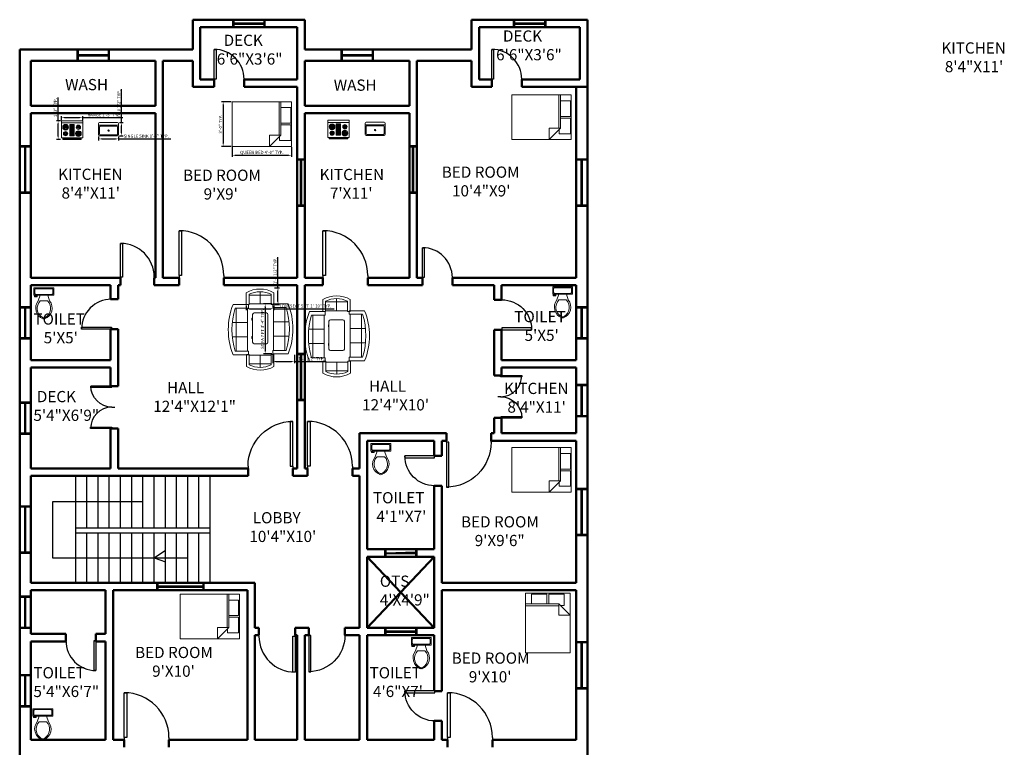
# Model space of a CAD drawing. Units: inches. Extents: x -31438 to -28352, y 12489 to 13610.
# Tile 5 of 5: x -29143 to -28352, y 13026 to 13610. Entities that reach past the tile are written whole.
import ezdxf

# ---------------------------------------------------------------- set-up
doc = ezdxf.new("R2010")
doc.units = ezdxf.units.IN
for name, color, linetype, lineweight in [('A-ANNO-DIMS', 2, 'Continuous', 18), ('A-AREA-IDEN', 3, 'Continuous', 18), ('A-DOOR', 3, 'Continuous', 25), ('A-FLOR-FIXT', 9, 'Continuous', 18), ('A-FLOR-STRS', 6, 'Continuous', 25), ('A-FURN', 8, 'Continuous', 18), ('A-GLAZ', 4, 'Continuous', 25), ('A-WALL', 7, 'Continuous', 50)]:
    doc.layers.add(name, color=color, linetype=linetype, lineweight=lineweight)
doc.styles.get("Standard").update_dxf_attribs({"font": 'arial.ttf'})
doc.dimstyles.new('ISO-25', dxfattribs={"dimtxt": 2.5, "dimasz": 2.5, "dimexe": 1.25, "dimexo": 0.625, "dimtad": 1, "dimdec": 0, "dimlunit": 3, "dimtxsty": 'Standard', "dimcen": 2.5, "dimadec": 0, "dimazin": 0, "dimtfac": 1, "dimtdec": 0, "dimtmove": 0, "dimatfit": 3, "dimfxl": 1, "dimarcsym": 0})

# ---------------------------------------------------------------- blocks, each defined once
blk = doc.blocks.new('*U8')
for p, q in [((0, 0), (0, -100)), ((750, 0), (750, -100))]:
    blk.add_line(p, q)
blk.add_lwpolyline([(0, 0), (0, 750), (43.75, 750), (43.75, 0)], close=True)
blk.add_arc((0, 0), 750, 0, 90)
blk = doc.blocks.new('Bed - Queen')
for p, q in [((0, -80.00003), (0, 0)), ((0, 0), (59.99999, 0)), ((59.99999, 0), (59.99999, -80.00003)), ((7.99999, -1.2), (28.79998, -1.2)), ((7.99999, -14.4), (7.99999, -1.2)), ((28.79998, -1.2), (28.79998, -14.4)), ((31.19999, -1.2), (51.99999, -1.2)), ((31.19999, -14.4), (31.19999, -1.2)), ((51.99999, -1.2), (51.99999, -16.4)), ((0, -14.4), (44.8, -14.4)), ((44.8, -16.8), (0, -16.8)), ((59.99999, -29.6), (44.8, -14.4)), ((44.8, -14.4), (44.8, -29.6)), ((51.99999, -16.4), (46.79936, -16.4)), ((44.8, -29.6), (59.99999, -29.6)), ((59.99999, -80.00003), (0, -80.00003))]:
    blk.add_line(p, q)
blk = doc.blocks.new('Desk - 30 x 60 in.')
for p, q in [((-26.999995, 0), (26.999995, 0)), ((-29.999995, -27), (-29.999995, -3)), ((29.999995, -3), (29.999995, -27)), ((26.999995, -30), (-26.999995, -30)), ((-20.000005, -30), (-20.000005, -31)), ((-20.000005, -31), (-16.000005, -31)), ((-16.000005, -31), (-16.000005, -30)), ((15.999995, -31), (15.999995, -30)), ((19.999995, -31), (15.999995, -31)), ((19.999995, -30), (19.999995, -31))]:
    blk.add_line(p, q)
for centre, start, end in [((-26.499995, -3.5), 98.1301, 171.8699), ((26.499995, -3.5), 8.130102, 81.8699), ((-26.499995, -26.5), 188.1301, 261.8699), ((26.499995, -26.5), 278.1301, 351.8699)]:
    blk.add_arc(centre, 3.535534, start, end)
blk = doc.blocks.new('Sofa - Roundback 7 ft.')
for p, q in [((-36.000027, -34), (-36.000027, -11.4696)), ((-35.999844, -13.3819), (35.9998, -13.3819)), ((-12.00002, -32.4421), (-12.00003, -6.5971)), ((11.99997, -32.4421), (11.99998, -6.5971)), ((35.99998, -34), (35.99998, -11.4696)), ((-36.000027, -32.4421), (35.99998, -32.4421))]:
    blk.add_line(p, q)
for points in [[(-36.000027, -34), (-42.000027, -34), (-42.000027, -8)], [(41.99998, -8), (41.99998, -34), (35.99998, -34)]]:
    blk.add_lwpolyline(points)
for centre, radius, start, end in [((0, -114.25), 114.25, 68.43141, 111.5686), ((-0.00001, -127.1968), 121.1968, 72.72033, 107.2797)]:
    blk.add_arc(centre, radius, start, end)
blk = doc.blocks.new('Sofa - Roundback Loveseat 5 ft.')
for p, q in [((-24, -33.99998), (-24, -11.46958)), ((-23.9998, -13.38178), (23.99986, -13.38178)), ((0, -32.44198), (0, -5.99998)), ((24.00004, -33.99998), (24.00004, -11.46958)), ((-24, -32.44198), (24.00004, -32.44198))]:
    blk.add_line(p, q)
for points in [[(-24, -33.99998), (-30, -33.99998), (-30, -7.99998)], [(30.00004, -7.99998), (30.00004, -33.99998), (24.00004, -33.99998)]]:
    blk.add_lwpolyline(points)
for centre, radius, start, end in [((0, -60.24998), 60.24998, 60.13715, 119.8628), ((0, -61.38438), 55.38444, 64.32083, 115.6792)]:
    blk.add_arc(centre, radius, start, end)
blk = doc.blocks.new('Toilet - top')
for p, q in [((-10, -8.5), (-8, -8.5)), ((-10, -9.5), (-10, -8.5)), ((-7, -9.5), (-10, -9.5)), ((-8, -8.5), (-8, -8)), ((-7, -8), (-7, -9.5)), ((-4, -8), (-6, -14)), ((4, -8), (6, -14)), ((9.5, -6), (9.5, -2)), ((4, -14), (-4, -14))]:
    blk.add_line(p, q)
blk.add_lwpolyline([(10.5, -8), (10.5, 0), (-10.5, 0), (-10.5, -8)], close=True)
for points in [[(-9.5, -2), (-9.5, -6)], [(8.5, -1), (-8.5, -1)], [(-8.5, -7), (8.5, -7)]]:
    blk.add_lwpolyline(points)
for centre, radius, start, end in [((-8.6, -1.9), 0.884, 81.8699, 188.1301), ((-8.6, -6.1), 0.884, 171.8699, 278.1301), ((8.6, -1.9), 0.884, 351.8699, 98.1301), ((8.6, -6.1), 0.884, 261.8699, 8.1301), ((3.5, -21.6), 12.2, 141.4691, 247.9714), ((4.2, -21.8), 11.3, 136.3677, 238.9468), ((-3.5, -21.6), 12.2, 292.0284, 38.5307), ((-4.2, -21.8), 11.3, 301.053, 43.6321), ((0, -27.9), 4, 245.7318, 294.2682), ((0, -29), 4, 254.8605, 285.1395)]:
    blk.add_arc(centre, radius, start, end)
blk = doc.blocks.new('Range-Oven - 30 in top')
for p, q in [((0, -3), (30, -3)), ((12, -6), (18, -6)), ((13, -20), (13, -6)), ((14, -6), (14, -20)), ((15, -20), (15, -6)), ((16, -6), (16, -20)), ((17, -20), (17, -6)), ((6, -24), (6, -25)), ((8, -25), (8, -24)), ((18, -20), (12, -20)), ((22, -25), (22, -24)), ((24, -24), (24, -25))]:
    blk.add_line(p, q)
for points in [[(0, -24), (0, 0), (30, 0), (30, -24)], [(12, -21), (12, -5), (18, -5), (18, -21)], [(2, -26), (2, -25), (28, -25), (28, -26)]]:
    blk.add_lwpolyline(points, close=True)
for centre, radius in [((6, -9), 4), ((6, -9), 3), ((6, -9), 2), ((6, -9), 1), ((24, -9), 3), ((24, -9), 2), ((24, -9), 1), ((6, -18), 3), ((6, -18), 2), ((6, -18), 1), ((24, -18), 4), ((24, -18), 3), ((24, -18), 2), ((24, -18), 1)]:
    blk.add_circle(centre, radius)
blk = doc.blocks.new('Sink-single - 30 in top')
blk.add_line((-15, -3.999996), (15, -3.999996))
for points in [[(-13.5, 0), (13.5, 0)], [(-15, -18.499996), (-15, -1.5)], [(-13.5, -17.499996), (-13.5, -6.499996)], [(-12.5, -5.499996), (12.5, -5.499996)], [(13.5, -6.499996), (13.5, -17.499996)], [(15, -1.5), (15, -18.499996)], [(13.5, -19.999996), (-13.5, -19.999996)], [(12.5, -18.499996), (-12.5, -18.499996)]]:
    blk.add_lwpolyline(points)
for radius in [1, 0.5]:
    blk.add_circle((0, -11.999996), radius)
for centre, radius, start, end in [((-13.5, -1.5), 1.5, 90, 180), ((-12.5, -6.499996), 1, 90, 180), ((12.5, -6.499996), 1, 0, 90), ((13.5, -1.5), 1.5, 0, 90), ((-13.5, -18.499996), 1.5, 180, 270), ((-12.5, -17.499996), 1, 180, 270), ((12.5, -17.499996), 1, 270, 0), ((13.5, -18.499996), 1.5, 270, 0)]:
    blk.add_arc(centre, radius, start, end)
blk = doc.blocks.new('WIN-24')
for p, q in [((0, 0), (0, 24)), ((0.5, 0), (0.5, 24))]:
    blk.add_line(p, q)
blk = doc.blocks.new('WIN-36')
for p, q in [((0, 0), (0, 36)), ((0.5, 0), (0.5, 36))]:
    blk.add_line(p, q)
blk = doc.blocks.new('*D179')
at = {"layer": 'A-ANNO-DIMS', "color": 0, "lineweight": -2, "transparency": 16777216}
for p, q in [((-28940.39, 13381.63), (-28947.04, 13381.63)), ((-28945.79, 13379.13), (-28945.79, 13343.94)), ((-28940.39, 13341.44), (-28947.04, 13341.44))]:
    blk.add_line(p, q, dxfattribs=at)
at = {"layer": 'A-ANNO-DIMS', "color": 0, "transparency": 16777216}
for points in [[(-28946.21, 13379.13), (-28945.38, 13379.13), (-28945.79, 13381.63)], [(-28946.21, 13343.94), (-28945.38, 13343.94), (-28945.79, 13341.44)]]:
    blk.add_solid(points, dxfattribs=at)
at = {"layer": 'Defpoints', "color": 0, "transparency": 16777216}
for p in [(-28939.77, 13381.63), (-28945.79, 13341.44), (-28939.77, 13341.44)]:
    blk.add_point(p, dxfattribs=at)
at = {"layer": 'A-ANNO-DIMS', "color": 0, "transparency": 16777216, "insert": (-28947.71, 13361.54), "char_height": 2.5, "attachment_point": 5, "rotation": 90}
blk.add_mtext('SOFA 7 FT 3\'-4" TYP.', dxfattribs=at)
blk = doc.blocks.new('*D180')
at = {"layer": 'A-ANNO-DIMS', "color": 0, "lineweight": -2, "transparency": 16777216}
for p, q in [((-28939.77, 13340.82), (-28939.77, 13334.17)), ((-28937.27, 13335.42), (-28924.73, 13335.42)), ((-28922.23, 13340.82), (-28922.23, 13334.17)), ((-28922.23, 13335.42), (-28897.65, 13335.42))]:
    blk.add_line(p, q, dxfattribs=at)
at = {"layer": 'A-ANNO-DIMS', "color": 0, "transparency": 16777216}
for points in [[(-28937.27, 13335.83), (-28937.27, 13335), (-28939.77, 13335.42)], [(-28924.73, 13335.83), (-28924.73, 13335), (-28922.23, 13335.42)]]:
    blk.add_solid(points, dxfattribs=at)
at = {"layer": 'Defpoints', "color": 0, "transparency": 16777216}
for p in [(-28939.77, 13341.44), (-28922.23, 13341.44), (-28922.23, 13335.42)]:
    blk.add_point(p, dxfattribs=at)
at = {"layer": 'A-ANNO-DIMS', "color": 0, "transparency": 16777216, "insert": (-28908.69, 13337.33), "char_height": 2.5, "attachment_point": 5}
blk.add_mtext('1\'-5 1/2" TYP.', dxfattribs=at)
blk = doc.blocks.new('*D183')
at = {"layer": 'A-ANNO-DIMS', "color": 0, "lineweight": -2, "transparency": 16777216}
for p, q in [((-28960.97, 13380.44), (-28960.97, 13376.5)), ((-28958.47, 13377.75), (-28941.37, 13377.75)), ((-28938.87, 13380.44), (-28938.87, 13376.5)), ((-28938.87, 13377.75), (-28890.49, 13377.75))]:
    blk.add_line(p, q, dxfattribs=at)
at = {"layer": 'A-ANNO-DIMS', "color": 0, "transparency": 16777216}
for points in [[(-28958.47, 13378.17), (-28958.47, 13377.33), (-28960.97, 13377.75)], [(-28941.37, 13378.17), (-28941.37, 13377.33), (-28938.87, 13377.75)]]:
    blk.add_solid(points, dxfattribs=at)
at = {"layer": 'Defpoints', "color": 0, "transparency": 16777216}
for p in [(-28960.97, 13381.06), (-28938.87, 13381.06), (-28938.87, 13377.75)]:
    blk.add_point(p, dxfattribs=at)
at = {"layer": 'A-ANNO-DIMS', "color": 0, "transparency": 16777216, "insert": (-28913.43, 13379.67), "char_height": 2.5, "attachment_point": 5}
blk.add_mtext('LOVESEAT 5 FT 1\'-10" TYP.', dxfattribs=at)
blk = doc.blocks.new('*D184')
at = {"layer": 'A-ANNO-DIMS', "color": 0, "lineweight": -2, "transparency": 16777216}
for p, q in [((-28935.56, 13394.57), (-28935.56, 13419.14)), ((-28938.25, 13394.57), (-28934.31, 13394.57)), ((-28935.56, 13383.56), (-28935.56, 13392.07)), ((-28938.25, 13381.06), (-28934.31, 13381.06))]:
    blk.add_line(p, q, dxfattribs=at)
at = {"layer": 'A-ANNO-DIMS', "color": 0, "transparency": 16777216}
for points in [[(-28935.98, 13392.07), (-28935.14, 13392.07), (-28935.56, 13394.57)], [(-28935.98, 13383.56), (-28935.14, 13383.56), (-28935.56, 13381.06)]]:
    blk.add_solid(points, dxfattribs=at)
at = {"layer": 'Defpoints', "color": 0, "transparency": 16777216}
for p in [(-28938.87, 13394.57), (-28935.56, 13394.57), (-28938.87, 13381.06)]:
    blk.add_point(p, dxfattribs=at)
at = {"layer": 'A-ANNO-DIMS', "color": 0, "transparency": 16777216, "insert": (-28937.48, 13408.11), "char_height": 2.5, "attachment_point": 5, "rotation": 90}
blk.add_mtext('1\'-1 1/2" TYP.', dxfattribs=at)
blk = doc.blocks.new('*D187')
at = {"layer": 'A-ANNO-DIMS', "color": 0, "lineweight": -2, "transparency": 16777216}
for p, q in [((-28972.38, 13507.49), (-28972.38, 13499.69)), ((-28969.88, 13500.94), (-28927.09, 13500.94)), ((-28924.59, 13507.49), (-28924.59, 13499.69))]:
    blk.add_line(p, q, dxfattribs=at)
at = {"layer": 'A-ANNO-DIMS', "color": 0, "transparency": 16777216}
for points in [[(-28969.88, 13501.36), (-28969.88, 13500.53), (-28972.38, 13500.94)], [(-28927.09, 13501.36), (-28927.09, 13500.53), (-28924.59, 13500.94)]]:
    blk.add_solid(points, dxfattribs=at)
at = {"layer": 'Defpoints', "color": 0, "transparency": 16777216}
for p in [(-28972.38, 13508.11), (-28924.59, 13508.11), (-28924.59, 13500.94)]:
    blk.add_point(p, dxfattribs=at)
at = {"layer": 'A-ANNO-DIMS', "color": 0, "transparency": 16777216, "insert": (-28948.48, 13502.94), "char_height": 2.5, "attachment_point": 5}
blk.add_mtext('QUEEN BED 4\'-0" TYP.', dxfattribs=at)
blk = doc.blocks.new('*D188')
at = {"layer": 'A-ANNO-DIMS', "color": 0, "lineweight": -2, "transparency": 16777216}
for p, q in [((-28973, 13543.95), (-28980.8, 13543.95)), ((-28979.55, 13541.45), (-28979.55, 13510.61)), ((-28973, 13508.11), (-28980.8, 13508.11))]:
    blk.add_line(p, q, dxfattribs=at)
at = {"layer": 'A-ANNO-DIMS', "color": 0, "transparency": 16777216}
for points in [[(-28979.96, 13541.45), (-28979.13, 13541.45), (-28979.55, 13543.95)], [(-28979.96, 13510.61), (-28979.13, 13510.61), (-28979.55, 13508.11)]]:
    blk.add_solid(points, dxfattribs=at)
at = {"layer": 'Defpoints', "color": 0, "transparency": 16777216}
for p in [(-28972.38, 13543.95), (-28979.55, 13508.11), (-28972.38, 13508.11)]:
    blk.add_point(p, dxfattribs=at)
at = {"layer": 'A-ANNO-DIMS', "color": 0, "transparency": 16777216, "insert": (-28981.45, 13526.03), "char_height": 2.5, "attachment_point": 5, "rotation": 90}
blk.add_mtext('3\'-0" TYP.', dxfattribs=at)
blk = doc.blocks.new('*D199')
at = {"layer": 'A-ANNO-DIMS', "color": 0, "lineweight": -2, "transparency": 16777216}
for p, q in [((-29109.53, 13529.21), (-29109.53, 13532.4)), ((-29092.38, 13529.21), (-29092.38, 13532.4)), ((-29107.03, 13531.15), (-29094.88, 13531.15)), ((-29092.38, 13531.15), (-29060.13, 13531.15))]:
    blk.add_line(p, q, dxfattribs=at)
at = {"layer": 'A-ANNO-DIMS', "color": 0, "transparency": 16777216}
for points in [[(-29107.03, 13531.57), (-29107.03, 13530.74), (-29109.53, 13531.15)], [(-29094.88, 13531.57), (-29094.88, 13530.74), (-29092.38, 13531.15)]]:
    blk.add_solid(points, dxfattribs=at)
at = {"layer": 'Defpoints', "color": 0, "transparency": 16777216}
for p in [(-29109.53, 13528.58), (-29092.38, 13531.15), (-29092.38, 13528.58)]:
    blk.add_point(p, dxfattribs=at)
at = {"layer": 'A-ANNO-DIMS', "color": 0, "transparency": 16777216, "insert": (-29075.01, 13533.07), "char_height": 2.5, "attachment_point": 5}
blk.add_mtext('RANGE 1\'-5" TYP.', dxfattribs=at)
blk = doc.blocks.new('*D200')
at = {"layer": 'A-ANNO-DIMS', "color": 0, "lineweight": -2, "transparency": 16777216}
for p, q in [((-29112.1, 13528.58), (-29112.1, 13547.34)), ((-29110.16, 13528.58), (-29113.35, 13528.58)), ((-29112.1, 13516.22), (-29112.1, 13526.08)), ((-29110.16, 13513.72), (-29113.35, 13513.72))]:
    blk.add_line(p, q, dxfattribs=at)
at = {"layer": 'A-ANNO-DIMS', "color": 0, "transparency": 16777216}
for points in [[(-29112.52, 13526.08), (-29111.69, 13526.08), (-29112.1, 13528.58)], [(-29112.52, 13516.22), (-29111.69, 13516.22), (-29112.1, 13513.72)]]:
    blk.add_solid(points, dxfattribs=at)
at = {"layer": 'Defpoints', "color": 0, "transparency": 16777216}
for p in [(-29112.1, 13528.58), (-29109.53, 13528.58), (-29109.53, 13513.72)]:
    blk.add_point(p, dxfattribs=at)
at = {"layer": 'A-ANNO-DIMS', "color": 0, "transparency": 16777216, "insert": (-29114.01, 13539.21), "char_height": 2.5, "attachment_point": 5, "rotation": 90}
blk.add_mtext('1\'-3" TYP.', dxfattribs=at)
blk = doc.blocks.new('*D207')
at = {"layer": 'A-ANNO-DIMS', "color": 0, "lineweight": -2, "transparency": 16777216}
for p, q in [((-29079.59, 13515.87), (-29079.59, 13512.84)), ((-29077.09, 13514.09), (-29066.07, 13514.09)), ((-29063.57, 13515.87), (-29063.57, 13512.84)), ((-29063.57, 13514.09), (-29021.69, 13514.09))]:
    blk.add_line(p, q, dxfattribs=at)
at = {"layer": 'A-ANNO-DIMS', "color": 0, "transparency": 16777216}
for points in [[(-29077.09, 13514.51), (-29077.09, 13513.68), (-29079.59, 13514.09)], [(-29066.07, 13514.51), (-29066.07, 13513.68), (-29063.57, 13514.09)]]:
    blk.add_solid(points, dxfattribs=at)
at = {"layer": 'Defpoints', "color": 0, "transparency": 16777216}
for p in [(-29079.59, 13516.5), (-29063.57, 13516.5), (-29063.57, 13514.09)]:
    blk.add_point(p, dxfattribs=at)
at = {"layer": 'A-ANNO-DIMS', "color": 0, "transparency": 16777216, "insert": (-29041.38, 13516.01), "char_height": 2.5, "attachment_point": 5}
blk.add_mtext('SINGLE SINK 1\'-4" TYP.', dxfattribs=at)
blk = doc.blocks.new('*D208')
at = {"layer": 'A-ANNO-DIMS', "color": 0, "lineweight": -2, "transparency": 16777216}
for p, q in [((-29061.16, 13527.18), (-29061.16, 13553.94)), ((-29062.94, 13527.18), (-29059.91, 13527.18)), ((-29061.16, 13519), (-29061.16, 13524.68)), ((-29062.94, 13516.5), (-29059.91, 13516.5))]:
    blk.add_line(p, q, dxfattribs=at)
at = {"layer": 'A-ANNO-DIMS', "color": 0, "transparency": 16777216}
for points in [[(-29061.58, 13524.68), (-29060.74, 13524.68), (-29061.16, 13527.18)], [(-29061.58, 13519), (-29060.74, 13519), (-29061.16, 13516.5)]]:
    blk.add_solid(points, dxfattribs=at)
at = {"layer": 'Defpoints', "color": 0, "transparency": 16777216}
for p in [(-29063.57, 13527.18), (-29061.16, 13527.18), (-29063.57, 13516.5)]:
    blk.add_point(p, dxfattribs=at)
at = {"layer": 'A-ANNO-DIMS', "color": 0, "transparency": 16777216, "insert": (-29063.08, 13541.81), "char_height": 2.5, "attachment_point": 5, "rotation": 90}
blk.add_mtext('0\'-10 1/2" TYP.', dxfattribs=at)

msp = doc.modelspace()

# ---------------------------------------------------------------- linework, layer by layer
at = {"layer": 'A-FLOR-STRS'}
for p, q in [((-29097.99, 13157.75), (-29097.99, 13243.55)), ((-29088.99, 13201.75), (-29088.99, 13243.55)), ((-29079.99, 13201.75), (-29079.99, 13243.55)), ((-29070.99, 13201.75), (-29070.99, 13243.55)), ((-29061.99, 13201.75), (-29061.99, 13243.55)), ((-29052.99, 13201.75), (-29052.99, 13243.55)), ((-29043.99, 13201.75), (-29043.99, 13243.55)), ((-29034.99, 13201.75), (-29034.99, 13243.55)), ((-29025.99, 13201.75), (-29025.99, 13243.55)), ((-29016.99, 13201.75), (-29016.99, 13243.55)), ((-29007.99, 13201.75), (-29007.99, 13243.55)), ((-28998.99, 13201.75), (-28998.99, 13243.55)), ((-28989.99, 13157.75), (-28989.99, 13243.55)), ((-29043.99, 13222.65), (-29116.64, 13222.65)), ((-29116.64, 13222.65), (-29116.64, 13177.75)), ((-28989.99, 13201.75), (-29097.99, 13201.75)), ((-28989.99, 13197.75), (-29097.99, 13197.75)), ((-29088.99, 13157.75), (-29088.99, 13197.75)), ((-29079.99, 13157.75), (-29079.99, 13197.75)), ((-29070.99, 13157.75), (-29070.99, 13197.75)), ((-29061.99, 13157.75), (-29061.99, 13197.75)), ((-29052.99, 13157.75), (-29052.99, 13197.75)), ((-29043.99, 13157.75), (-29043.99, 13197.75)), ((-29034.99, 13157.75), (-29034.99, 13197.75)), ((-29025.99, 13157.75), (-29025.99, 13197.75)), ((-29016.99, 13157.75), (-29016.99, 13197.75)), ((-29007.99, 13157.75), (-29007.99, 13197.75)), ((-28998.99, 13157.75), (-28998.99, 13197.75)), ((-29116.64, 13177.75), (-29007.99, 13177.75)), ((-29034.99, 13177.75), (-29025.99, 13183.92)), ((-29034.99, 13177.75), (-29025.99, 13174.61))]:
    msp.add_line(p, q, dxfattribs=at)
at = {"layer": 'A-GLAZ'}
for p, q in [((-28971.99, 13609.75), (-28971.99, 13603.75)), ((-28970.99, 13609.75), (-28970.99, 13603.75)), ((-28970.99, 13607.25), (-28946.99, 13607.25)), ((-28970.99, 13606.75), (-28946.99, 13606.75)), ((-28970.99, 13606.25), (-28946.99, 13606.25)), ((-28946.99, 13609.75), (-28946.99, 13603.75)), ((-28945.99, 13609.75), (-28945.99, 13603.75)), ((-28746.49, 13609.75), (-28746.49, 13603.75)), ((-28745.49, 13609.75), (-28745.49, 13603.75)), ((-28745.49, 13607.25), (-28721.49, 13607.25)), ((-28745.49, 13606.75), (-28721.49, 13606.75)), ((-28745.49, 13606.25), (-28721.49, 13606.25)), ((-28721.49, 13609.75), (-28721.49, 13603.75)), ((-28720.49, 13609.75), (-28720.49, 13603.75)), ((-29096.99, 13585.75), (-29096.99, 13576.75)), ((-29095.99, 13585.75), (-29095.99, 13576.75)), ((-29095.99, 13581.75), (-29071.99, 13581.75)), ((-29095.99, 13581.25), (-29071.99, 13581.25)), ((-29095.99, 13580.75), (-29071.99, 13580.75)), ((-29071.99, 13585.75), (-29071.99, 13576.75)), ((-29070.99, 13585.75), (-29070.99, 13576.75)), ((-28884.99, 13585.75), (-28884.99, 13576.75)), ((-28883.99, 13585.75), (-28883.99, 13576.75)), ((-28883.99, 13581.75), (-28859.99, 13581.75)), ((-28883.99, 13581.25), (-28859.99, 13581.25)), ((-28883.99, 13580.75), (-28859.99, 13580.75)), ((-28859.99, 13585.75), (-28859.99, 13576.75)), ((-28858.99, 13585.75), (-28858.99, 13576.75)), ((-29142.99, 13508.65), (-29133.99, 13508.65)), ((-28829.99, 13508.65), (-28823.99, 13508.65)), ((-29142.99, 13507.65), (-29133.99, 13507.65)), ((-29138.99, 13471.65), (-29138.99, 13507.65)), ((-29138.49, 13471.65), (-29138.49, 13507.65)), ((-29137.99, 13471.65), (-29137.99, 13507.65)), ((-28829.99, 13507.65), (-28823.99, 13507.65)), ((-28827.49, 13471.65), (-28827.49, 13507.65)), ((-28826.99, 13471.65), (-28826.99, 13507.65)), ((-28826.49, 13471.65), (-28826.49, 13507.65)), ((-28919.99, 13498.15), (-28913.99, 13498.15)), ((-28919.99, 13497.15), (-28913.99, 13497.15)), ((-28917.49, 13461.15), (-28917.49, 13497.15)), ((-28916.99, 13461.15), (-28916.99, 13497.15)), ((-28916.49, 13461.15), (-28916.49, 13497.15)), ((-28695.99, 13498.15), (-28686.99, 13498.15)), ((-28695.99, 13497.15), (-28686.99, 13497.15)), ((-28691.99, 13461.15), (-28691.99, 13497.15)), ((-28691.49, 13461.15), (-28691.49, 13497.15)), ((-28690.99, 13461.15), (-28690.99, 13497.15)), ((-29142.99, 13471.65), (-29133.99, 13471.65)), ((-29142.99, 13470.65), (-29133.99, 13470.65)), ((-28829.99, 13471.65), (-28823.99, 13471.65)), ((-28829.99, 13470.65), (-28823.99, 13470.65)), ((-28919.99, 13461.15), (-28913.99, 13461.15)), ((-28695.99, 13461.15), (-28686.99, 13461.15)), ((-28919.99, 13460.15), (-28913.99, 13460.15)), ((-28695.99, 13460.15), (-28686.99, 13460.15)), ((-29142.99, 13379.55), (-29133.99, 13379.55)), ((-29142.99, 13378.55), (-29133.99, 13378.55)), ((-29138.99, 13354.55), (-29138.99, 13378.55)), ((-29138.49, 13354.55), (-29138.49, 13378.55)), ((-29137.99, 13354.55), (-29137.99, 13378.55)), ((-28695.99, 13379.55), (-28686.99, 13379.55)), ((-28695.99, 13378.55), (-28686.99, 13378.55)), ((-28691.99, 13354.55), (-28691.99, 13378.55)), ((-28691.49, 13354.55), (-28691.49, 13378.55)), ((-28690.99, 13354.55), (-28690.99, 13378.55)), ((-29142.99, 13354.55), (-29133.99, 13354.55)), ((-29142.99, 13353.55), (-29133.99, 13353.55)), ((-28695.99, 13354.55), (-28686.99, 13354.55)), ((-28695.99, 13353.55), (-28686.99, 13353.55)), ((-28919.99, 13342.05), (-28913.99, 13342.05)), ((-28919.99, 13341.05), (-28913.99, 13341.05)), ((-28917.49, 13305.05), (-28917.49, 13341.05)), ((-28916.99, 13305.05), (-28916.99, 13341.05)), ((-28916.49, 13305.05), (-28916.49, 13341.05)), ((-28695.99, 13317.15), (-28686.99, 13317.15)), ((-28695.99, 13316.15), (-28686.99, 13316.15)), ((-28691.99, 13292.15), (-28691.99, 13316.15)), ((-28691.49, 13292.15), (-28691.49, 13316.15)), ((-28690.99, 13292.15), (-28690.99, 13316.15)), ((-29142.99, 13303.05), (-29133.99, 13303.05)), ((-28919.99, 13305.05), (-28913.99, 13305.05)), ((-28919.99, 13304.05), (-28913.99, 13304.05)), ((-29142.99, 13302.05), (-29133.99, 13302.05)), ((-29138.99, 13278.05), (-29138.99, 13302.05)), ((-29138.49, 13278.05), (-29138.49, 13302.05)), ((-29137.99, 13278.05), (-29137.99, 13302.05)), ((-28695.99, 13292.15), (-28686.99, 13292.15)), ((-28695.99, 13291.15), (-28686.99, 13291.15)), ((-29142.99, 13278.05), (-29133.99, 13278.05)), ((-29142.99, 13277.05), (-29133.99, 13277.05)), ((-28695.99, 13233.75), (-28686.99, 13233.75)), ((-28695.99, 13232.75), (-28686.99, 13232.75)), ((-28691.99, 13196.75), (-28691.99, 13232.75)), ((-28691.49, 13196.75), (-28691.49, 13232.75)), ((-28690.99, 13196.75), (-28690.99, 13232.75)), ((-29142.99, 13219.65), (-29133.99, 13219.65)), ((-29142.99, 13218.65), (-29133.99, 13218.65)), ((-29138.99, 13182.65), (-29138.99, 13218.65)), ((-29138.49, 13182.65), (-29138.49, 13218.65)), ((-29137.99, 13182.65), (-29137.99, 13218.65)), ((-28695.99, 13196.75), (-28686.99, 13196.75)), ((-28695.99, 13195.75), (-28686.99, 13195.75)), ((-28849.99, 13184.75), (-28849.99, 13178.75)), ((-28848.99, 13184.75), (-28848.99, 13178.75)), ((-28824.99, 13184.75), (-28824.99, 13178.75)), ((-28823.99, 13184.75), (-28823.99, 13178.75)), ((-29142.99, 13182.65), (-29133.99, 13182.65)), ((-29142.99, 13181.65), (-29133.99, 13181.65)), ((-28848.99, 13181.25), (-28824.99, 13181.25)), ((-29032.99, 13157.75), (-29032.99, 13151.75)), ((-29031.99, 13157.75), (-29031.99, 13151.75)), ((-29031.99, 13155.25), (-28995.99, 13155.25)), ((-28995.99, 13157.75), (-28995.99, 13151.75)), ((-28994.99, 13157.75), (-28994.99, 13151.75)), ((-29142.99, 13147.25), (-29133.99, 13147.25)), ((-29142.99, 13146.25), (-29133.99, 13146.25)), ((-29138.99, 13122.25), (-29138.99, 13146.25)), ((-29138.49, 13122.25), (-29138.49, 13146.25)), ((-29137.99, 13122.25), (-29137.99, 13146.25)), ((-29142.99, 13122.25), (-29133.99, 13122.25)), ((-29142.99, 13121.25), (-29133.99, 13121.25)), ((-28849.99, 13121.75), (-28849.99, 13115.75)), ((-28848.99, 13121.75), (-28848.99, 13115.75)), ((-28824.99, 13121.75), (-28824.99, 13115.75)), ((-28823.99, 13121.75), (-28823.99, 13115.75)), ((-28848.99, 13119.25), (-28824.99, 13119.25)), ((-28848.99, 13118.75), (-28824.99, 13118.75)), ((-28848.99, 13118.25), (-28824.99, 13118.25)), ((-28695.99, 13110.75), (-28686.99, 13110.75)), ((-28695.99, 13109.75), (-28686.99, 13109.75)), ((-28691.99, 13073.75), (-28691.99, 13109.75)), ((-28691.49, 13073.75), (-28691.49, 13109.75)), ((-28690.99, 13073.75), (-28690.99, 13109.75)), ((-29142.99, 13084.25), (-29133.99, 13084.25)), ((-29142.99, 13083.25), (-29133.99, 13083.25)), ((-29138.99, 13059.25), (-29138.99, 13083.25)), ((-29138.49, 13059.25), (-29138.49, 13083.25)), ((-29137.99, 13059.25), (-29137.99, 13083.25)), ((-28695.99, 13073.75), (-28686.99, 13073.75)), ((-28695.99, 13072.75), (-28686.99, 13072.75)), ((-29142.99, 13059.25), (-29133.99, 13059.25)), ((-29142.99, 13058.25), (-29133.99, 13058.25))]:
    msp.add_line(p, q, dxfattribs=at)
at = {"layer": 'A-WALL'}
for p, q in [((-29003.99, 13609.75), (-28913.99, 13609.75)), ((-29003.99, 13585.75), (-29003.99, 13609.75)), ((-28997.99, 13603.75), (-28919.99, 13603.75)), ((-28997.99, 13561.75), (-28997.99, 13603.75)), ((-28919.99, 13561.75), (-28919.99, 13603.75)), ((-28913.99, 13585.75), (-28913.99, 13609.75)), ((-28779.99, 13609.75), (-28686.99, 13609.75)), ((-28779.99, 13609.75), (-28779.99, 13585.75)), ((-28773.99, 13603.75), (-28692.99, 13603.75)), ((-28773.99, 13603.75), (-28773.99, 13561.75)), ((-28692.99, 13603.75), (-28692.99, 13561.75)), ((-28686.99, 13609.75), (-28686.99, 12745.75)), ((-29142.99, 13585.75), (-29003.99, 13585.75)), ((-29142.99, 12721.75), (-29142.99, 13585.75)), ((-28913.99, 13585.75), (-28779.99, 13585.75)), ((-29133.99, 13576.75), (-29033.99, 13576.75)), ((-29133.99, 13540.75), (-29133.99, 13576.75)), ((-29033.99, 13540.75), (-29033.99, 13576.75)), ((-29027.99, 13576.75), (-29003.99, 13576.75)), ((-29027.99, 13402.55), (-29027.99, 13576.75)), ((-29003.99, 13555.75), (-29003.99, 13576.75)), ((-28913.99, 13576.75), (-28829.99, 13576.75)), ((-28913.99, 13540.75), (-28913.99, 13576.75)), ((-28829.99, 13540.75), (-28829.99, 13576.75)), ((-28823.99, 13576.75), (-28779.99, 13576.75)), ((-28823.99, 13402.55), (-28823.99, 13576.75)), ((-28779.99, 13576.75), (-28779.99, 13555.75)), ((-28997.99, 13561.75), (-28986.71, 13561.75)), ((-28986.71, 13561.75), (-28986.71, 13555.75)), ((-28962.71, 13561.75), (-28919.99, 13561.75)), ((-28962.71, 13561.75), (-28962.71, 13555.75)), ((-28773.99, 13561.75), (-28763.75, 13561.75)), ((-28763.75, 13561.75), (-28763.75, 13555.75)), ((-28739.75, 13561.75), (-28692.99, 13561.75)), ((-28739.75, 13561.75), (-28739.75, 13555.75)), ((-29003.99, 13555.75), (-28986.71, 13555.75)), ((-28962.71, 13555.75), (-28919.99, 13555.75)), ((-28919.99, 13402.55), (-28919.99, 13555.75)), ((-28779.99, 13555.75), (-28763.75, 13555.75)), ((-28739.75, 13555.75), (-28686.99, 13555.75)), ((-28695.99, 13555.75), (-28695.99, 13402.55)), ((-29133.99, 13540.75), (-29033.99, 13540.75)), ((-28913.99, 13540.75), (-28829.99, 13540.75)), ((-29133.99, 13534.75), (-29033.99, 13534.75)), ((-29133.99, 13402.55), (-29133.99, 13534.75)), ((-29033.99, 13402.55), (-29033.99, 13534.75)), ((-28913.99, 13534.75), (-28829.99, 13534.75)), ((-28913.99, 13402.55), (-28913.99, 13534.75)), ((-28829.99, 13402.55), (-28829.99, 13534.75)), ((-29061.94, 13402.55), (-29133.99, 13402.55)), ((-29061.94, 13402.55), (-29061.94, 13396.55)), ((-29033.99, 13402.55), (-29034.94, 13402.55)), ((-29034.94, 13402.55), (-29034.94, 13396.55)), ((-29014.99, 13402.55), (-29027.99, 13402.55)), ((-29014.99, 13402.55), (-29014.99, 13396.55)), ((-28919.99, 13402.55), (-28978.99, 13402.55)), ((-28978.99, 13402.55), (-28978.99, 13396.55)), ((-28899.37, 13402.55), (-28913.99, 13402.55)), ((-28899.37, 13402.55), (-28899.37, 13396.55)), ((-28829.99, 13402.55), (-28863.37, 13402.55)), ((-28863.37, 13402.55), (-28863.37, 13396.55)), ((-28819.47, 13402.55), (-28823.99, 13402.55)), ((-28819.47, 13402.55), (-28819.47, 13396.55)), ((-28695.99, 13402.55), (-28795.47, 13402.55)), ((-28795.47, 13402.55), (-28795.47, 13396.55)), ((-29133.99, 13336.55), (-29133.99, 13396.55)), ((-29069.99, 13396.55), (-29133.99, 13396.55)), ((-29069.99, 13385.41), (-29069.99, 13396.55)), ((-29063.99, 13385.41), (-29063.99, 13396.55)), ((-29061.94, 13396.55), (-29063.99, 13396.55)), ((-29014.99, 13396.55), (-29034.94, 13396.55)), ((-28919.99, 13396.55), (-28978.99, 13396.55)), ((-28919.99, 13249.55), (-28919.99, 13396.55)), ((-28913.99, 13249.55), (-28913.99, 13396.55)), ((-28899.37, 13396.55), (-28913.99, 13396.55)), ((-28819.47, 13396.55), (-28863.37, 13396.55)), ((-28761.99, 13396.55), (-28795.47, 13396.55)), ((-28761.99, 13396.55), (-28761.99, 13384.9)), ((-28755.99, 13396.55), (-28755.99, 13384.9)), ((-28695.99, 13396.55), (-28755.99, 13396.55)), ((-28695.99, 13396.55), (-28695.99, 13336.55)), ((-29069.99, 13385.41), (-29063.99, 13385.41)), ((-28761.99, 13384.9), (-28755.99, 13384.9)), ((-29069.99, 13336.55), (-29069.99, 13361.41)), ((-29069.99, 13361.41), (-29063.99, 13361.41)), ((-29063.99, 13315.73), (-29063.99, 13361.41)), ((-28761.99, 13360.9), (-28761.99, 13324.11)), ((-28761.99, 13360.9), (-28755.99, 13360.9)), ((-28755.99, 13360.9), (-28755.99, 13336.55)), ((-29069.99, 13336.55), (-29133.99, 13336.55)), ((-28695.99, 13336.55), (-28755.99, 13336.55)), ((-29133.99, 13249.55), (-29133.99, 13330.55)), ((-29069.99, 13330.55), (-29133.99, 13330.55)), ((-29069.99, 13315.73), (-29069.99, 13330.55)), ((-28755.99, 13330.55), (-28755.99, 13324.11)), ((-28695.99, 13330.55), (-28755.99, 13330.55)), ((-28695.99, 13330.55), (-28695.99, 13277.75)), ((-28761.99, 13324.11), (-28755.99, 13324.11)), ((-29069.99, 13315.73), (-29063.99, 13315.73)), ((-28761.99, 13290.11), (-28761.99, 13277.75)), ((-28761.99, 13290.11), (-28755.99, 13290.11)), ((-28755.99, 13290.11), (-28755.99, 13277.75)), ((-29069.99, 13249.55), (-29069.99, 13281.73)), ((-29069.99, 13281.73), (-29063.99, 13281.73)), ((-29063.99, 13249.55), (-29063.99, 13281.73)), ((-28869.99, 13277.75), (-28869.99, 13249.55)), ((-28800.28, 13277.75), (-28869.99, 13277.75)), ((-28863.99, 13271.75), (-28863.99, 13184.75)), ((-28809.99, 13271.75), (-28863.99, 13271.75)), ((-28809.99, 13271.75), (-28809.99, 13259.67)), ((-28803.99, 13271.75), (-28803.99, 13259.67)), ((-28800.28, 13271.75), (-28803.99, 13271.75)), ((-28800.28, 13277.75), (-28800.28, 13271.75)), ((-28761.99, 13277.75), (-28764.28, 13277.75)), ((-28764.28, 13277.75), (-28764.28, 13271.75)), ((-28695.99, 13271.75), (-28764.28, 13271.75)), ((-28695.99, 13277.75), (-28755.99, 13277.75)), ((-28695.99, 13271.75), (-28695.99, 13157.75)), ((-28809.99, 13259.67), (-28803.99, 13259.67)), ((-29069.99, 13249.55), (-29133.99, 13249.55)), ((-28959.55, 13249.55), (-29063.99, 13249.55)), ((-28959.55, 13249.55), (-28959.55, 13243.55)), ((-28919.99, 13249.55), (-28923.55, 13249.55)), ((-28923.55, 13249.55), (-28923.55, 13243.55)), ((-28911.78, 13249.55), (-28913.99, 13249.55)), ((-28911.78, 13249.55), (-28911.78, 13243.55)), ((-28869.99, 13249.55), (-28875.78, 13249.55)), ((-28875.78, 13249.55), (-28875.78, 13243.55)), ((-29133.99, 13157.75), (-29133.99, 13243.55)), ((-28959.55, 13243.55), (-29133.99, 13243.55)), ((-28911.78, 13243.55), (-28923.55, 13243.55)), ((-28869.99, 13243.55), (-28875.78, 13243.55)), ((-28869.99, 13243.55), (-28869.99, 13121.75)), ((-28809.99, 13235.67), (-28809.99, 13184.75)), ((-28809.99, 13235.67), (-28803.99, 13235.67)), ((-28803.99, 13235.67), (-28803.99, 13157.75)), ((-28809.99, 13184.75), (-28863.99, 13184.75)), ((-28863.99, 13178.75), (-28863.99, 13121.75)), ((-28809.99, 13178.75), (-28863.99, 13178.75)), ((-28809.99, 13178.75), (-28863.99, 13121.75)), ((-28863.99, 13178.75), (-28809.99, 13121.75)), ((-28809.99, 13178.75), (-28809.99, 13121.75)), ((-28953.99, 13157.75), (-29133.99, 13157.75)), ((-28953.99, 13121.75), (-28953.99, 13157.75)), ((-28695.99, 13157.75), (-28803.99, 13157.75)), ((-29073.99, 13151.75), (-29133.99, 13151.75)), ((-29133.99, 13116.75), (-29133.99, 13151.75)), ((-29073.99, 13116.75), (-29073.99, 13151.75)), ((-28959.99, 13151.75), (-29067.99, 13151.75)), ((-29067.99, 13031.75), (-29067.99, 13151.75)), ((-28959.99, 13031.75), (-28959.99, 13151.75)), ((-28803.99, 13151.75), (-28803.99, 13070.87)), ((-28695.99, 13151.75), (-28803.99, 13151.75)), ((-28695.99, 13151.75), (-28695.99, 13031.75)), ((-28950.81, 13121.75), (-28953.99, 13121.75)), ((-28950.81, 13121.75), (-28950.81, 13115.75)), ((-28910.81, 13121.75), (-28921.81, 13121.75)), ((-28921.81, 13121.75), (-28921.81, 13115.75)), ((-28910.81, 13121.75), (-28910.81, 13115.75)), ((-28869.99, 13121.75), (-28881.81, 13121.75)), ((-28881.81, 13121.75), (-28881.81, 13115.75)), ((-28809.99, 13121.75), (-28863.99, 13121.75)), ((-29105.9, 13116.75), (-29133.99, 13116.75)), ((-29105.9, 13116.75), (-29105.9, 13110.75)), ((-29073.99, 13116.75), (-29081.9, 13116.75)), ((-29081.9, 13116.75), (-29081.9, 13110.75)), ((-28950.81, 13115.75), (-28953.99, 13115.75)), ((-28953.99, 13031.75), (-28953.99, 13115.75)), ((-28919.99, 13115.75), (-28921.81, 13115.75)), ((-28919.99, 13031.75), (-28919.99, 13115.75)), ((-28910.81, 13115.75), (-28913.99, 13115.75)), ((-28913.99, 13031.75), (-28913.99, 13115.75)), ((-28869.99, 13115.75), (-28881.81, 13115.75)), ((-28869.99, 13115.75), (-28869.99, 13031.75)), ((-28863.99, 13115.75), (-28863.99, 13031.75)), ((-28809.99, 13115.75), (-28863.99, 13115.75)), ((-28809.99, 13115.75), (-28809.99, 13070.87)), ((-29105.9, 13110.75), (-29133.99, 13110.75)), ((-29133.99, 13031.75), (-29133.99, 13110.75)), ((-29073.99, 13110.75), (-29081.9, 13110.75)), ((-29073.99, 13031.75), (-29073.99, 13110.75)), ((-28809.99, 13070.87), (-28803.99, 13070.87)), ((-28809.99, 13046.87), (-28809.99, 13031.75)), ((-28809.99, 13046.87), (-28803.99, 13046.87)), ((-28803.99, 13046.87), (-28803.99, 13031.75)), ((-29073.99, 13031.75), (-29133.99, 13031.75)), ((-29059.11, 13031.75), (-29067.99, 13031.75)), ((-29059.11, 13031.75), (-29059.11, 13025.75)), ((-28959.99, 13031.75), (-29023.11, 13031.75)), ((-29023.11, 13031.75), (-29023.11, 13025.75)), ((-28919.99, 13031.75), (-28953.99, 13031.75)), ((-28869.99, 13031.75), (-28913.99, 13031.75)), ((-28809.99, 13031.75), (-28863.99, 13031.75)), ((-28799.32, 13031.75), (-28803.99, 13031.75)), ((-28799.32, 13031.75), (-28799.32, 13025.75)), ((-28695.99, 13031.75), (-28763.32, 13031.75)), ((-28763.32, 13031.75), (-28763.32, 13025.75)), ((-28695.99, 13031.75), (-28761.99, 13031.75))]:
    msp.add_line(p, q, dxfattribs=at)

# ---------------------------------------------------------------- block references
at = {"layer": 'A-DOOR'}
for p, xscale, yscale, zscale in [((-28986.71, 13561.95), 0.0320000000000057, 0.0320000000000057, 0.0320000000000057), ((-28763.75, 13561.95), 0.0320000000000009, 0.0320000000000009, 0.0320000000000009), ((-29014.99, 13404.35), 0.0480000000000013, 0.0480000000000013, 0.0480000000000013), ((-28899.37, 13404.35), 0.0480000000000062, 0.0480000000000062, 0.0480000000000062), ((-29061.94, 13403.15), 0.036000000000001, 0.036000000000001, 0.036000000000001), ((-28819.47, 13402.75), 0.031999999999996, 0.031999999999996, 0.031999999999996), ((-28923.55, 13251.35), -0.0480000000000062, 0.0480000000000062, 0.0480000000000062), ((-28911.78, 13251.35), 0.0480000000000062, 0.0480000000000062, 0.0480000000000062), ((-29059.11, 13033.55), 0.0480000000000013, 0.0480000000000013, 0.0480000000000013), ((-28799.32, 13033.55), 0.0480000000000062, 0.0480000000000062, 0.0480000000000062)]:
    msp.add_blockref('*U8', p, dxfattribs=dict(at, xscale=xscale, yscale=yscale, zscale=zscale))
for p, xscale, yscale, zscale, rotation in [((-29069.36, 13361.47), 0.0319309066466794, 0.0319309066466794, 0.0319309066466794, 90.00000000000003), ((-28755.79, 13360.9), -0.032000000296522, 0.032000000296522, 0.032000000296522, 270), ((-28756.73, 13324.12), 0.022636277250161, 0.022636277250161, 0.022636277250161, 270), ((-29068.89, 13315.73), -0.022636277250161, 0.022636277250161, 0.022636277250161, 90), ((-28756.57, 13290.11), -0.022666666666667, 0.022666666666667, 0.022666666666667, 270), ((-29069.06, 13281.72), 0.022666666666667, 0.022666666666667, 0.022666666666667, 90.00000000000003), ((-28800.27, 13270.64), -0.0480000000000062, 0.0480000000000062, 0.0480000000000062, 180), ((-28809.71, 13259.56), -0.031855356978981, 0.031855356978981, 0.031855356978981, 90), ((-29081.9, 13111.39), 0.0319999999999995, 0.0319999999999995, 0.0319999999999995, 180), ((-28921.83, 13115.03), 0.0386429077113226, 0.0386429077113226, 0.0386429077113226, 180), ((-28910.81, 13115.44), -0.0386666666666638, 0.0386666666666638, 0.0386666666666638, 180), ((-28809.42, 13070.97), -0.0321317879517036, 0.0321317879517036, 0.0321317879517036, 90)]:
    msp.add_blockref('*U8', p, dxfattribs=dict(at, xscale=xscale, yscale=yscale, zscale=zscale, rotation=rotation))
at = {"layer": 'A-FLOR-FIXT'}
for name, p, xscale, yscale, zscale in [('Range-Oven - 30 in top', (-29109.53, 13528.58), 0.5716393668778607, 0.5716393668778607, 0.5716393668778607), ('Sink-single - 30 in top', (-29071.58, 13527.18), 0.534256555286997, 0.534256555286997, 0.534256555286997), ('Range-Oven - 30 in top', (-28895.52, 13528.99), 0.5716393668778607, 0.5716393668778607, 0.5716393668778607), ('Sink-single - 30 in top', (-28857.57, 13527.59), 0.534256555286997, 0.534256555286997, 0.534256555286997), ('Toilet - top', (-29123.55, 13394.62), 0.7575755229467699, 0.7575755229467699, 0.7575755229467699), ('Toilet - top', (-28706.93, 13395.41), 0.7575755229467699, 0.7575755229467699, 0.7575755229467699), ('Toilet - top', (-28852.93, 13269.57), 0.7575755229467699, 0.7575755229467699, 0.7575755229467699), ('Toilet - top', (-28820.45, 13113.76), 0.7575755229467699, 0.7575755229467699, 0.7575755229467699), ('Toilet - top', (-29124.38, 13056.75), 0.7575755229467699, 0.7575755229467699, 0.7575755229467699)]:
    msp.add_blockref(name, p, dxfattribs=dict(at, xscale=xscale, yscale=yscale, zscale=zscale))
at = {"layer": 'A-FURN'}
for name, p, xscale, yscale, zscale, rotation in [('Bed - Queen', (-28699.95, 13549.33), 0.597358992664269, 0.597358992664269, 0.597358992664269, 270), ('Bed - Queen', (-28924.59, 13543.95), 0.597358992664269, 0.597358992664269, 0.597358992664269, 270), ('Sofa - Roundback 7 ft.', (-28975.44, 13360.97), 0.4784035434924597, 0.4784035434924597, 0.4784035434924597, 89.99999999999999), ('Desk - 30 x 60 in.', (-28943.61, 13362.02), 0.4130441003592061, 0.4130441003592061, 0.4130441003592061, 270), ('Sofa - Roundback 7 ft.', (-28923.5, 13361.54), 0.4784035434924597, 0.4784035434924597, 0.4784035434924597, 270), ('Sofa - Roundback 7 ft.', (-28914.01, 13355.49), 0.4784035434924597, 0.4784035434924597, 0.4784035434924597, 89.99999999999999), ('Sofa - Roundback 7 ft.', (-28862.07, 13356.06), 0.4784035434924597, 0.4784035434924597, 0.4784035434924597, 270), ('Desk - 30 x 60 in.', (-28882.17, 13356.55), 0.4130441003592061, 0.4130441003592061, 0.4130441003592061, 270), ('Sofa - Roundback Loveseat 5 ft.', (-28949.79, 13328.51), 0.3682442798772706, 0.3682442798772706, 0.3682442798772706, 180), ('Sofa - Roundback Loveseat 5 ft.', (-28888.36, 13323.04), 0.3682442798772706, 0.3682442798772706, 0.3682442798772706, 180), ('Bed - Queen', (-28699.97, 13266.29), 0.597358992664269, 0.597358992664269, 0.597358992664269, 270), ('Bed - Queen', (-28966.4, 13148.73), 0.597358992664269, 0.597358992664269, 0.597358992664269, 270)]:
    msp.add_blockref(name, p, dxfattribs=dict(at, xscale=xscale, yscale=yscale, zscale=zscale, rotation=rotation))
for name, p, xscale, yscale, zscale in [('Sofa - Roundback Loveseat 5 ft.', (-28949.92, 13393.58), 0.3682442798772706, 0.3682442798772706, 0.3682442798772706), ('Sofa - Roundback Loveseat 5 ft.', (-28888.49, 13388.11), 0.3682442798772706, 0.3682442798772706, 0.3682442798772706), ('Bed - Queen', (-28736.65, 13149.43), 0.597358992664269, 0.597358992664269, 0.597358992664269)]:
    msp.add_blockref(name, p, dxfattribs=dict(at, xscale=xscale, yscale=yscale, zscale=zscale))
at = {"layer": 'A-GLAZ'}
for name, p, rotation in [('WIN-24', (-28848.99, 13181.75), 272.3869788479644), ('WIN-36', (-29031.99, 13154.75), 269.9999999999997)]:
    msp.add_blockref(name, p, dxfattribs=dict(at, rotation=rotation))

# ---------------------------------------------------------------- texts
at = {"layer": 'A-AREA-IDEN', "char_height": 9, "attachment_point": 1}
for s, insert in [('{  DECK\\P6\'6"X3\'6"}', (-28984.68, 13597.71)), ('{  DECK\\P6\'6"X3\'6"}', (-28760.32, 13601.16)), ('{KITCHEN\\P 8\'4"X11\'}', (-28402.63, 13591.57)), ('{WASH}', (-29106.52, 13562.16)), ('{WASH}', (-28890.75, 13561.74)), ('{KITCHEN\\P 8\'4"X11\'}', (-29112.13, 13490.19)), ("{BED ROOM\\P      9'X9'}", (-29011.75, 13489.41)), ("{KITCHEN\\P   7'X11'}", (-28902.09, 13489.98)), ('{BED ROOM\\P   10\'4"X9\'}', (-28803.97, 13491.91)), ("{TOILET\\P   5'X5'}", (-29131.97, 13374.02)), ("{   TOILET\\P      5'X5'}", (-28753.97, 13375.94)), ('{    HALL\\P12\'4"X12\'1"}', (-29035.69, 13318.92)), ('{    HALL\\P  12\'4"X10\'}', (-28873.43, 13320.13)), ('{ DECK\\P5\'4"X6\'9"}', (-29131.97, 13311.74)), ('{KITCHEN\\P 8\'4"X11\'}', (-28753.97, 13318.32)), ('{ TOILET\\P  4\'1"X7\'}', (-28861.97, 13230.57)), ('{ LOBBY\\P10\'4"X10\'}', (-28958.51, 13214.51)), ('{BED ROOM\\P    9\'X9\'6"}', (-28788.51, 13211.22)), ('{   OTS\\P   4\'X4\'9"}', (-28861.97, 13163.55)), ("{BED ROOM\\P     9'X10'}", (-29050.34, 13106.37)), ("{BED ROOM\\P     9'X10'}", (-28796, 13101.84)), ('{TOILET\\P5\'4"X6\'7"}', (-29131.97, 13090.08)), ('{TOILET\\P 4\'6"X7\'}', (-28861.97, 13090.08))]:
    msp.add_mtext_dynamic_manual_height_columns(s, width=772.4312, gutter_width=12.5, heights=[0], dxfattribs=dict(at, insert=insert))

# ---------------------------------------------------------------- dimensions: what is measured, and where the dimension line sits
at = {"layer": 'A-ANNO-DIMS'}
for base, p1, p2, angle, text, picture, middle in [((-29061.16, 13527.18), (-29063.57, 13516.5), (-29063.57, 13527.18), 90, '<> TYP.', '*D208', (-29063.08, 13541.81)), ((-29112.1, 13528.58), (-29109.53, 13513.72), (-29109.53, 13528.58), 90, '<> TYP.', '*D200', (-29114.01, 13539.21)), ((-28979.55, 13508.11), (-28972.38, 13543.95), (-28972.38, 13508.11), 270, '<> TYP.', '*D188', (-28981.45, 13526.03)), ((-28935.56, 13394.57), (-28938.87, 13381.06), (-28938.87, 13394.57), 90, '<> TYP.', '*D184', (-28937.48, 13408.11)), ((-28945.79, 13341.44), (-28939.77, 13381.63), (-28939.77, 13341.44), 270, 'SOFA 7 FT <> TYP.', '*D179', (-28947.71, 13361.54))]:
    dim = msp.add_linear_dim(base=base, p1=p1, p2=p2, angle=angle, text=text, dimstyle='ISO-25', override={"dimdec": 1, "dimlfac": 1, "dimrnd": 0, "dimzin": 1, "dimdsep": 46, "dimlunit": 4, "dimfrac": 2}, dxfattribs=at)
    dim.commit()
    dim.dimension.update_dxf_attribs({"geometry": picture, "text_midpoint": middle})
for base, p1, p2, text, picture, middle in [((-29092.3813, 13531.1546), (-29109.5304, 13528.5822), (-29092.3813, 13528.5822), 'RANGE <> TYP.', '*D199', (-29075.0066, 13533.0722)), ((-29063.57, 13514.09), (-29079.59, 13516.5), (-29063.57, 13516.5), 'SINGLE SINK <> TYP.', '*D207', (-29041.38, 13516.01)), ((-28924.59, 13500.94), (-28972.38, 13508.11), (-28924.59, 13508.11), 'QUEEN BED <> TYP.', '*D187', (-28948.48, 13502.94)), ((-28938.87, 13377.75), (-28960.97, 13381.06), (-28938.87, 13381.06), 'LOVESEAT 5 FT <> TYP.', '*D183', (-28913.43, 13379.67)), ((-28922.23, 13335.42), (-28939.77, 13341.44), (-28922.23, 13341.44), '<> TYP.', '*D180', (-28908.69, 13337.33))]:
    dim = msp.add_linear_dim(base=base, p1=p1, p2=p2, text=text, dimstyle='ISO-25', override={"dimdec": 1, "dimlfac": 1, "dimrnd": 0, "dimzin": 1, "dimdsep": 46, "dimlunit": 4, "dimfrac": 2}, dxfattribs=at)
    dim.commit()
    dim.dimension.update_dxf_attribs({"geometry": picture, "text_midpoint": middle})

doc.saveas('drawing.dxf')
